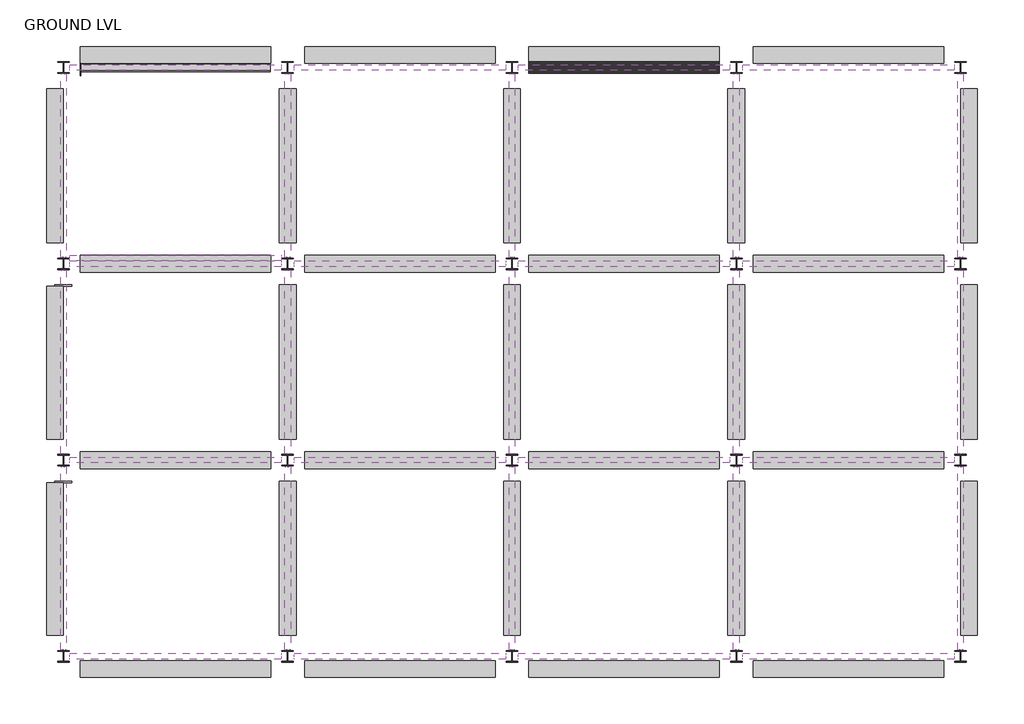
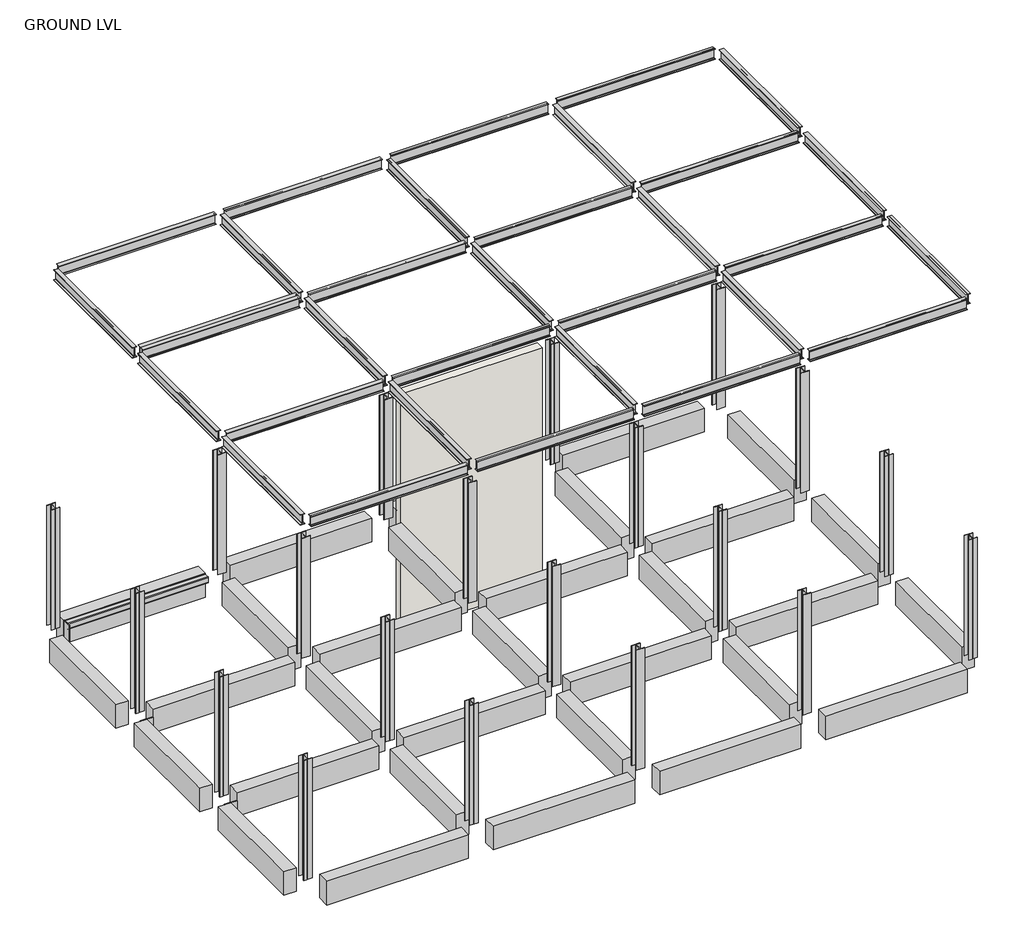
# One storey: 67 beams, 20 columns, 1 wall.
"""IFC4 building model written with IfcOpenShell, lengths in millimetres."""

from ifc_helpers import new_model, si_unit, frame, origin, place, context, project, spatial, polyline, outline, extrude, faceted_brep, transform, mapped, element, save
from components import m_hss_square_hss152_4x152_4x9_5_4d3a2309, ub_universal_beams_ub254x102x28_022e5764, ub_universal_beams_ub254x102x28_3359efaf, ub_universal_beams_ub254x102x28_3001bc84, uc_universal_columns_column_uc203x203x52_f24fe326

model = new_model("IFC4")

# Units and contexts
model_context = context("Model", 3, world=origin())
ifc_project = project(units=[si_unit("LENGTHUNIT", "METRE", prefix="MILLI")], contexts=[model_context])

# Site, building, storey
site = spatial("IfcSite", under=ifc_project)
building = spatial("IfcBuilding", under=site)
storey = spatial("IfcBuildingStorey", under=building, Name="GROUND LVL", Elevation=0.0)

# Beams
placement = place(None, origin())
element("IfcBeam", 1, ObjectType="M_Concrete-Rectangular Beam : 300 x 600mm", at=placement, inside=storey, context=model_context, shape_type="Brep", body=[
    faceted_brep([(-5230.6620752, 9930.8028699, 0.0), (-5230.6620752, 10230.8028699, 0.0), (-8630.6620752, 10230.8028699, 0.0), (-8630.6620752, 9930.8028699, 0.0), (-8617.9620752, 9930.8028699, 0.0), (-5230.6620752, 9930.8028699, -600.0), (-8630.6620752, 9930.8028699, -600.0), (-8617.9620752, 9930.8028699, -600.0), (-5230.6620752, 10230.8028699, -600.0), (-8630.6620752, 10230.8028699, -600.0)], [[[0, 1, 2, 3, 4]], [[5, 0, 4, 3, 6, 7]], [[8, 5, 7, 6, 9]], [[1, 8, 9, 2]], [[2, 9, 6, 3]], [[1, 0, 5, 8]]]),
])
element("IfcBeam", 2, ObjectType="M_Concrete-Rectangular Beam : 300 x 600mm", at=placement, inside=storey, context=model_context, shape_type="SweptSolid", body=[
    extrude(outline(polyline([(-1230.6620752, 10230.8028699), (-1230.6620752, 9930.8028699), (-4630.6620752, 9930.8028699), (-4630.6620752, 10230.8028699), (-1230.6620752, 10230.8028699)])), frame((0.0, 0.0, -600.0), z_axis=(0.0, 0.0, 1.0), x_axis=(1.0, 0.0, 0.0)), (0.0, 0.0, 1.0), 600.0),
])
element("IfcBeam", 3, ObjectType="M_Concrete-Rectangular Beam : 300 x 600mm", at=placement, inside=storey, context=model_context, shape_type="SweptSolid", body=[
    extrude(outline(polyline([(-8930.6620752, 6730.8028699), (-9230.6620752, 6730.8028699), (-9230.6620752, 9480.8028699), (-8930.6620752, 9480.8028699), (-8930.6620752, 6730.8028699)])), frame((0.0, 0.0, -600.0), z_axis=(0.0, 0.0, 1.0), x_axis=(1.0, 0.0, 0.0)), (0.0, 0.0, 1.0), 600.0),
])
element("IfcBeam", 4, ObjectType="M_Concrete-Rectangular Beam : 300 x 600mm", at=placement, inside=storey, context=model_context, shape_type="Brep", body=[
    faceted_brep([(-9230.6620752, 3230.8028699, 0.0), (-8930.6620752, 3230.8028699, 0.0), (-8930.6620752, 5955.8028699, 0.0), (-9080.6620752, 5955.8028699, 0.0), (-9230.6620752, 5955.8028699, 0.0), (-9230.6620752, 3230.8028699, -600.0), (-9230.6620752, 5955.8028699, -600.0), (-8930.6620752, 3230.8028699, -600.0), (-9080.6620752, 5955.8028699, -600.0), (-8930.6620752, 5955.8028699, -600.0)], [[[0, 1, 2, 3, 4]], [[5, 0, 4, 6]], [[7, 5, 6, 8, 9]], [[1, 7, 9, 2]], [[2, 9, 8, 6, 4, 3]], [[1, 0, 5, 7]]]),
])
element("IfcBeam", 5, ObjectType="M_Concrete-Rectangular Beam : 300 x 600mm", at=placement, inside=storey, context=model_context, shape_type="Brep", body=[
    faceted_brep([(-9230.6620752, -269.1971301, 0.0), (-8930.6620752, -269.1971301, 0.0), (-8930.6620752, 2455.8028699, 0.0), (-9080.6620752, 2455.8028699, 0.0), (-9230.6620752, 2455.8028699, 0.0), (-9230.6620752, -269.1971301, -600.0), (-9230.6620752, 2455.8028699, -600.0), (-8930.6620752, -269.1971301, -600.0), (-9080.6620752, 2455.8028699, -600.0), (-8930.6620752, 2455.8028699, -600.0)], [[[0, 1, 2, 3, 4]], [[5, 0, 4, 6]], [[7, 5, 6, 8, 9]], [[1, 7, 9, 2]], [[2, 9, 8, 6, 4, 3]], [[1, 0, 5, 7]]]),
])
element("IfcBeam", 6, ObjectType="M_Concrete-Rectangular Beam : 300 x 600mm", at=placement, inside=storey, context=model_context, shape_type="Brep", body=[
    faceted_brep([(-9080.6620752, 2455.8028699, 0.0), (-8930.6620752, 2455.8028699, 0.0), (-8780.6620752, 2455.8028699, 0.0), (-8780.6620752, 2480.8028699, 0.0), (-9080.6620752, 2480.8028699, 0.0), (-8780.6620752, 2455.8028699, -600.0), (-8780.6620752, 2480.8028699, -600.0), (-8930.6620752, 2455.8028699, -600.0), (-9080.6620752, 2455.8028699, -600.0), (-9080.6620752, 2480.8028699, -600.0)], [[[0, 1, 2, 3, 4]], [[2, 5, 6, 3]], [[5, 7, 8, 9, 6]], [[8, 0, 4, 9]], [[0, 8, 7, 5, 2, 1]], [[4, 3, 6, 9]]]),
])
element("IfcBeam", 7, ObjectType="M_Concrete-Rectangular Beam : 300 x 600mm", at=placement, inside=storey, context=model_context, shape_type="Brep", body=[
    faceted_brep([(-9080.6620752, 5955.8028699, 0.0), (-8930.6620752, 5955.8028699, 0.0), (-8780.6620752, 5955.8028699, 0.0), (-8780.6620752, 5980.8028699, 0.0), (-9080.6620752, 5980.8028699, 0.0), (-8780.6620752, 5955.8028699, -600.0), (-8780.6620752, 5980.8028699, -600.0), (-8930.6620752, 5955.8028699, -600.0), (-9080.6620752, 5955.8028699, -600.0), (-9080.6620752, 5980.8028699, -600.0)], [[[0, 1, 2, 3, 4]], [[2, 5, 6, 3]], [[5, 7, 8, 9, 6]], [[8, 0, 4, 9]], [[0, 8, 7, 5, 2, 1]], [[4, 3, 6, 9]]]),
])
element("IfcBeam", 8, ObjectType="M_Concrete-Rectangular Beam : 300 x 600mm", at=placement, inside=storey, context=model_context, shape_type="SweptSolid", body=[
    extrude(outline(polyline([(-5080.6620752, 2480.8028699), (-4780.6620752, 2480.8028699), (-4780.6620752, -269.1971301), (-5080.6620752, -269.1971301), (-5080.6620752, 2480.8028699)])), frame((0.0, 0.0, -600.0), z_axis=(0.0, 0.0, 1.0), x_axis=(1.0, 0.0, 0.0)), (0.0, 0.0, 1.0), 600.0),
])
element("IfcBeam", 9, ObjectType="M_Concrete-Rectangular Beam : 300 x 600mm", at=placement, inside=storey, context=model_context, shape_type="SweptSolid", body=[
    extrude(outline(polyline([(-5080.6620752, 5980.8028699), (-4780.6620752, 5980.8028699), (-4780.6620752, 3230.8028699), (-5080.6620752, 3230.8028699), (-5080.6620752, 5980.8028699)])), frame((0.0, 0.0, -600.0), z_axis=(0.0, 0.0, 1.0), x_axis=(1.0, 0.0, 0.0)), (0.0, 0.0, 1.0), 600.0),
])
element("IfcBeam", 10, ObjectType="M_Concrete-Rectangular Beam : 300 x 600mm", at=placement, inside=storey, context=model_context, shape_type="SweptSolid", body=[
    extrude(outline(polyline([(-5080.6620752, 9480.8028699), (-4780.6620752, 9480.8028699), (-4780.6620752, 6730.8028699), (-5080.6620752, 6730.8028699), (-5080.6620752, 9480.8028699)])), frame((0.0, 0.0, -600.0), z_axis=(0.0, 0.0, 1.0), x_axis=(1.0, 0.0, 0.0)), (0.0, 0.0, 1.0), 600.0),
])
element("IfcBeam", 11, ObjectType="M_Concrete-Rectangular Beam : 300 x 600mm", at=placement, inside=storey, context=model_context, shape_type="SweptSolid", body=[
    extrude(outline(polyline([(-1080.6620752, 2480.8028699), (-780.6620752, 2480.8028699), (-780.6620752, -269.1971301), (-1080.6620752, -269.1971301), (-1080.6620752, 2480.8028699)])), frame((0.0, 0.0, -600.0), z_axis=(0.0, 0.0, 1.0), x_axis=(1.0, 0.0, 0.0)), (0.0, 0.0, 1.0), 600.0),
])
element("IfcBeam", 12, ObjectType="M_Concrete-Rectangular Beam : 300 x 600mm", at=placement, inside=storey, context=model_context, shape_type="SweptSolid", body=[
    extrude(outline(polyline([(-1080.6620752, 5980.8028699), (-780.6620752, 5980.8028699), (-780.6620752, 3230.8028699), (-1080.6620752, 3230.8028699), (-1080.6620752, 5980.8028699)])), frame((0.0, 0.0, -600.0), z_axis=(0.0, 0.0, 1.0), x_axis=(1.0, 0.0, 0.0)), (0.0, 0.0, 1.0), 600.0),
])
element("IfcBeam", 13, ObjectType="M_Concrete-Rectangular Beam : 300 x 600mm", at=placement, inside=storey, context=model_context, shape_type="SweptSolid", body=[
    extrude(outline(polyline([(-1080.6620752, 9480.8028699), (-780.6620752, 9480.8028699), (-780.6620752, 6730.8028699), (-1080.6620752, 6730.8028699), (-1080.6620752, 9480.8028699)])), frame((0.0, 0.0, -600.0), z_axis=(0.0, 0.0, 1.0), x_axis=(1.0, 0.0, 0.0)), (0.0, 0.0, 1.0), 600.0),
])
element("IfcBeam", 14, ObjectType="M_Concrete-Rectangular Beam : 300 x 600mm", at=placement, inside=storey, context=model_context, shape_type="SweptSolid", body=[
    extrude(outline(polyline([(2919.3379248, 2480.8028699), (3219.3379248, 2480.8028699), (3219.3379248, -269.1971301), (2919.3379248, -269.1971301), (2919.3379248, 2480.8028699)])), frame((0.0, 0.0, -600.0), z_axis=(0.0, 0.0, 1.0), x_axis=(1.0, 0.0, 0.0)), (0.0, 0.0, 1.0), 600.0),
])
element("IfcBeam", 15, ObjectType="M_Concrete-Rectangular Beam : 300 x 600mm", at=placement, inside=storey, context=model_context, shape_type="SweptSolid", body=[
    extrude(outline(polyline([(2919.3379248, 5980.8028699), (3219.3379248, 5980.8028699), (3219.3379248, 3230.8028699), (2919.3379248, 3230.8028699), (2919.3379248, 5980.8028699)])), frame((0.0, 0.0, -600.0), z_axis=(0.0, 0.0, 1.0), x_axis=(1.0, 0.0, 0.0)), (0.0, 0.0, 1.0), 600.0),
])
element("IfcBeam", 16, ObjectType="M_Concrete-Rectangular Beam : 300 x 600mm", at=placement, inside=storey, context=model_context, shape_type="SweptSolid", body=[
    extrude(outline(polyline([(2919.3379248, 9480.8028699), (3219.3379248, 9480.8028699), (3219.3379248, 6730.8028699), (2919.3379248, 6730.8028699), (2919.3379248, 9480.8028699)])), frame((0.0, 0.0, -600.0), z_axis=(0.0, 0.0, 1.0), x_axis=(1.0, 0.0, 0.0)), (0.0, 0.0, 1.0), 600.0),
])
element("IfcBeam", 17, ObjectType="M_Concrete-Rectangular Beam : 300 x 600mm", at=placement, inside=storey, context=model_context, shape_type="SweptSolid", body=[
    extrude(outline(polyline([(7069.3379248, 2480.8028699), (7369.3379248, 2480.8028699), (7369.3379248, -269.1971301), (7069.3379248, -269.1971301), (7069.3379248, 2480.8028699)])), frame((0.0, 0.0, -600.0), z_axis=(0.0, 0.0, 1.0), x_axis=(1.0, 0.0, 0.0)), (0.0, 0.0, 1.0), 600.0),
])
element("IfcBeam", 18, ObjectType="M_Concrete-Rectangular Beam : 300 x 600mm", at=placement, inside=storey, context=model_context, shape_type="SweptSolid", body=[
    extrude(outline(polyline([(7069.3379248, 5980.8028699), (7369.3379248, 5980.8028699), (7369.3379248, 3230.8028699), (7069.3379248, 3230.8028699), (7069.3379248, 5980.8028699)])), frame((0.0, 0.0, -600.0), z_axis=(0.0, 0.0, 1.0), x_axis=(1.0, 0.0, 0.0)), (0.0, 0.0, 1.0), 600.0),
])
element("IfcBeam", 19, ObjectType="M_Concrete-Rectangular Beam : 300 x 600mm", at=placement, inside=storey, context=model_context, shape_type="SweptSolid", body=[
    extrude(outline(polyline([(7069.3379248, 9480.8028699), (7369.3379248, 9480.8028699), (7369.3379248, 6730.8028699), (7069.3379248, 6730.8028699), (7069.3379248, 9480.8028699)])), frame((0.0, 0.0, -600.0), z_axis=(0.0, 0.0, 1.0), x_axis=(1.0, 0.0, 0.0)), (0.0, 0.0, 1.0), 600.0),
])
element("IfcBeam", 20, ObjectType="M_Concrete-Rectangular Beam : 300 x 600mm", at=placement, inside=storey, context=model_context, shape_type="SweptSolid", body=[
    extrude(outline(polyline([(-8630.6620752, 9930.8028699), (-8617.9620752, 9930.8028699), (-8617.9620752, 9705.8028699), (-8630.6620752, 9705.8028699), (-8630.6620752, 9930.8028699)])), frame((0.0, 0.0, -600.0), z_axis=(0.0, 0.0, 1.0), x_axis=(1.0, 0.0, 0.0)), (0.0, 0.0, 1.0), 600.0),
])
element("IfcBeam", 21, ObjectType="M_Concrete-Rectangular Beam : 300 x 600mm", at=placement, inside=storey, context=model_context, shape_type="SweptSolid", body=[
    extrude(outline(polyline([(-630.6620752, 9930.8028699), (-630.6620752, 10230.8028699), (2769.3379248, 10230.8028699), (2769.3379248, 9930.8028699), (-630.6620752, 9930.8028699)])), frame((0.0, 0.0, -600.0), z_axis=(0.0, 0.0, 1.0), x_axis=(1.0, 0.0, 0.0)), (0.0, 0.0, 1.0), 600.0),
])
element("IfcBeam", 22, ObjectType="M_Concrete-Rectangular Beam : 300 x 600mm", at=placement, inside=storey, context=model_context, shape_type="SweptSolid", body=[
    extrude(outline(polyline([(3369.3379248, 9930.8028699), (3369.3379248, 10230.8028699), (6769.3379248, 10230.8028699), (6769.3379248, 9930.8028699), (3369.3379248, 9930.8028699)])), frame((0.0, 0.0, -600.0), z_axis=(0.0, 0.0, 1.0), x_axis=(1.0, 0.0, 0.0)), (0.0, 0.0, 1.0), 600.0),
])
element("IfcBeam", 23, ObjectType="M_Concrete-Rectangular Beam : 300 x 600mm", at=placement, inside=storey, context=model_context, shape_type="SweptSolid", body=[
    extrude(outline(polyline([(-8630.6620752, 6205.8028699), (-8630.6620752, 6505.8028699), (-5230.6620752, 6505.8028699), (-5230.6620752, 6205.8028699), (-8630.6620752, 6205.8028699)])), frame((0.0, 0.0, -600.0), z_axis=(0.0, 0.0, 1.0), x_axis=(1.0, 0.0, 0.0)), (0.0, 0.0, 1.0), 600.0),
])
element("IfcBeam", 24, ObjectType="M_Concrete-Rectangular Beam : 300 x 600mm", at=placement, inside=storey, context=model_context, shape_type="SweptSolid", body=[
    extrude(outline(polyline([(-4630.6620752, 6205.8028699), (-4630.6620752, 6505.8028699), (-1230.6620752, 6505.8028699), (-1230.6620752, 6205.8028699), (-4630.6620752, 6205.8028699)])), frame((0.0, 0.0, -600.0), z_axis=(0.0, 0.0, 1.0), x_axis=(1.0, 0.0, 0.0)), (0.0, 0.0, 1.0), 600.0),
])
element("IfcBeam", 25, ObjectType="M_Concrete-Rectangular Beam : 300 x 600mm", at=placement, inside=storey, context=model_context, shape_type="SweptSolid", body=[
    extrude(outline(polyline([(-630.6620752, 6205.8028699), (-630.6620752, 6505.8028699), (2769.3379248, 6505.8028699), (2769.3379248, 6205.8028699), (-630.6620752, 6205.8028699)])), frame((0.0, 0.0, -600.0), z_axis=(0.0, 0.0, 1.0), x_axis=(1.0, 0.0, 0.0)), (0.0, 0.0, 1.0), 600.0),
])
element("IfcBeam", 26, ObjectType="M_Concrete-Rectangular Beam : 300 x 600mm", at=placement, inside=storey, context=model_context, shape_type="SweptSolid", body=[
    extrude(outline(polyline([(3369.3379248, 6205.8028699), (3369.3379248, 6505.8028699), (6769.3379248, 6505.8028699), (6769.3379248, 6205.8028699), (3369.3379248, 6205.8028699)])), frame((0.0, 0.0, -600.0), z_axis=(0.0, 0.0, 1.0), x_axis=(1.0, 0.0, 0.0)), (0.0, 0.0, 1.0), 600.0),
])
element("IfcBeam", 27, ObjectType="M_Concrete-Rectangular Beam : 300 x 600mm", at=placement, inside=storey, context=model_context, shape_type="SweptSolid", body=[
    extrude(outline(polyline([(-8630.6620752, 2705.8028699), (-8630.6620752, 3005.8028699), (-5230.6620752, 3005.8028699), (-5230.6620752, 2705.8028699), (-8630.6620752, 2705.8028699)])), frame((0.0, 0.0, -600.0), z_axis=(0.0, 0.0, 1.0), x_axis=(1.0, 0.0, 0.0)), (0.0, 0.0, 1.0), 600.0),
])
element("IfcBeam", 28, ObjectType="M_Concrete-Rectangular Beam : 300 x 600mm", at=placement, inside=storey, context=model_context, shape_type="SweptSolid", body=[
    extrude(outline(polyline([(-4630.6620752, 2705.8028699), (-4630.6620752, 3005.8028699), (-1230.6620752, 3005.8028699), (-1230.6620752, 2705.8028699), (-4630.6620752, 2705.8028699)])), frame((0.0, 0.0, -600.0), z_axis=(0.0, 0.0, 1.0), x_axis=(1.0, 0.0, 0.0)), (0.0, 0.0, 1.0), 600.0),
])
element("IfcBeam", 29, ObjectType="M_Concrete-Rectangular Beam : 300 x 600mm", at=placement, inside=storey, context=model_context, shape_type="SweptSolid", body=[
    extrude(outline(polyline([(-630.6620752, 2705.8028699), (-630.6620752, 3005.8028699), (2769.3379248, 3005.8028699), (2769.3379248, 2705.8028699), (-630.6620752, 2705.8028699)])), frame((0.0, 0.0, -600.0), z_axis=(0.0, 0.0, 1.0), x_axis=(1.0, 0.0, 0.0)), (0.0, 0.0, 1.0), 600.0),
])
element("IfcBeam", 30, ObjectType="M_Concrete-Rectangular Beam : 300 x 600mm", at=placement, inside=storey, context=model_context, shape_type="SweptSolid", body=[
    extrude(outline(polyline([(3369.3379248, 2705.8028699), (3369.3379248, 3005.8028699), (6769.3379248, 3005.8028699), (6769.3379248, 2705.8028699), (3369.3379248, 2705.8028699)])), frame((0.0, 0.0, -600.0), z_axis=(0.0, 0.0, 1.0), x_axis=(1.0, 0.0, 0.0)), (0.0, 0.0, 1.0), 600.0),
])
element("IfcBeam", 31, ObjectType="M_Concrete-Rectangular Beam : 300 x 600mm", at=placement, inside=storey, context=model_context, shape_type="SweptSolid", body=[
    extrude(outline(polyline([(-8630.6620752, -1019.1971301), (-8630.6620752, -719.1971301), (-5230.6620752, -719.1971301), (-5230.6620752, -1019.1971301), (-8630.6620752, -1019.1971301)])), frame((0.0, 0.0, -600.0), z_axis=(0.0, 0.0, 1.0), x_axis=(1.0, 0.0, 0.0)), (0.0, 0.0, 1.0), 600.0),
])
element("IfcBeam", 32, ObjectType="M_Concrete-Rectangular Beam : 300 x 600mm", at=placement, inside=storey, context=model_context, shape_type="SweptSolid", body=[
    extrude(outline(polyline([(-4630.6620752, -1019.1971301), (-4630.6620752, -719.1971301), (-1230.6620752, -719.1971301), (-1230.6620752, -1019.1971301), (-4630.6620752, -1019.1971301)])), frame((0.0, 0.0, -600.0), z_axis=(0.0, 0.0, 1.0), x_axis=(1.0, 0.0, 0.0)), (0.0, 0.0, 1.0), 600.0),
])
element("IfcBeam", 33, ObjectType="M_Concrete-Rectangular Beam : 300 x 600mm", at=placement, inside=storey, context=model_context, shape_type="SweptSolid", body=[
    extrude(outline(polyline([(-630.6620752, -1019.1971301), (-630.6620752, -719.1971301), (2769.3379248, -719.1971301), (2769.3379248, -1019.1971301), (-630.6620752, -1019.1971301)])), frame((0.0, 0.0, -600.0), z_axis=(0.0, 0.0, 1.0), x_axis=(1.0, 0.0, 0.0)), (0.0, 0.0, 1.0), 600.0),
])
element("IfcBeam", 34, ObjectType="M_Concrete-Rectangular Beam : 300 x 600mm", at=placement, inside=storey, context=model_context, shape_type="SweptSolid", body=[
    extrude(outline(polyline([(3369.3379248, -1019.1971301), (3369.3379248, -719.1971301), (6769.3379248, -719.1971301), (6769.3379248, -1019.1971301), (3369.3379248, -1019.1971301)])), frame((0.0, 0.0, -600.0), z_axis=(0.0, 0.0, 1.0), x_axis=(1.0, 0.0, 0.0)), (0.0, 0.0, 1.0), 600.0),
])
m_hss_square_hss152_4x152_4x9_5_shape = m_hss_square_hss152_4x152_4x9_5_4d3a2309(model_context)
element("IfcBeam", 35, ObjectType="M_HSS Square : HSS152.4X152.4X9.5", at=placement, inside=storey, context=model_context, shape_type="MappedRepresentation", body=[
    mapped(m_hss_square_hss152_4x152_4x9_5_shape, transform((-6880.6620752, 9855.8028699, -76.0), x_axis=(1.0, 0.0, 0.0), y_axis=(0.0, 1.0, 0.0), z_axis=(0.0, 0.0, 1.0))),
])
ub_universal_beams_ub254x102x28_shape = ub_universal_beams_ub254x102x28_022e5764(model_context)
element("IfcBeam", 36, ObjectType="UB-Universal Beams : UB254x102x28", at=placement, inside=storey, context=model_context, shape_type="MappedRepresentation", body=[
    mapped(ub_universal_beams_ub254x102x28_shape, transform((-6871.2144105, 6458.2567898, 9013.8), x_axis=(1.0, 0.0, 0.0), y_axis=(0.0, 1.0, 0.0), z_axis=(0.0, 0.0, 1.0))),
])
ub_universal_beams_ub254x102x28_2_shape = ub_universal_beams_ub254x102x28_3359efaf(model_context)
element("IfcBeam", 37, ObjectType="UB-Universal Beams : UB254x102x28", at=placement, inside=storey, context=model_context, shape_type="MappedRepresentation", body=[
    mapped(ub_universal_beams_ub254x102x28_2_shape, transform((-8930.6620752, 1105.8028699, 9013.8), x_axis=(0.0, 1.0, 0.0), y_axis=(-1.0, 0.0, 0.0), z_axis=(0.0, 0.0, 1.0))),
])
element("IfcBeam", 38, ObjectType="UB-Universal Beams : UB254x102x28", at=placement, inside=storey, context=model_context, shape_type="MappedRepresentation", body=[
    mapped(ub_universal_beams_ub254x102x28_2_shape, transform((-8930.6620752, 4605.8028699, 9013.8), x_axis=(0.0, 1.0, 0.0), y_axis=(-1.0, 0.0, 0.0), z_axis=(0.0, 0.0, 1.0))),
])
element("IfcBeam", 39, ObjectType="UB-Universal Beams : UB254x102x28", at=placement, inside=storey, context=model_context, shape_type="MappedRepresentation", body=[
    mapped(ub_universal_beams_ub254x102x28_2_shape, transform((-8930.6620752, 8105.8028699, 9013.8), x_axis=(0.0, 1.0, 0.0), y_axis=(-1.0, 0.0, 0.0), z_axis=(0.0, 0.0, 1.0))),
])
element("IfcBeam", 40, ObjectType="UB-Universal Beams : UB254x102x28", at=placement, inside=storey, context=model_context, shape_type="MappedRepresentation", body=[
    mapped(ub_universal_beams_ub254x102x28_2_shape, transform((-4930.6620752, 1105.8028699, 9013.8), x_axis=(0.0, 1.0, 0.0), y_axis=(-1.0, 0.0, 0.0), z_axis=(0.0, 0.0, 1.0))),
])
element("IfcBeam", 41, ObjectType="UB-Universal Beams : UB254x102x28", at=placement, inside=storey, context=model_context, shape_type="MappedRepresentation", body=[
    mapped(ub_universal_beams_ub254x102x28_2_shape, transform((-4930.6620752, 4605.8028699, 9013.8), x_axis=(0.0, 1.0, 0.0), y_axis=(-1.0, 0.0, 0.0), z_axis=(0.0, 0.0, 1.0))),
])
element("IfcBeam", 42, ObjectType="UB-Universal Beams : UB254x102x28", at=placement, inside=storey, context=model_context, shape_type="MappedRepresentation", body=[
    mapped(ub_universal_beams_ub254x102x28_2_shape, transform((-4930.6620752, 8105.8028699, 9013.8), x_axis=(0.0, 1.0, 0.0), y_axis=(-1.0, 0.0, 0.0), z_axis=(0.0, 0.0, 1.0))),
])
element("IfcBeam", 43, ObjectType="UB-Universal Beams : UB254x102x28", at=placement, inside=storey, context=model_context, shape_type="MappedRepresentation", body=[
    mapped(ub_universal_beams_ub254x102x28_2_shape, transform((-930.6620752, 1105.8028699, 9013.8), x_axis=(0.0, 1.0, 0.0), y_axis=(-1.0, 0.0, 0.0), z_axis=(0.0, 0.0, 1.0))),
])
element("IfcBeam", 44, ObjectType="UB-Universal Beams : UB254x102x28", at=placement, inside=storey, context=model_context, shape_type="MappedRepresentation", body=[
    mapped(ub_universal_beams_ub254x102x28_2_shape, transform((-930.6620752, 4605.8028699, 9013.8), x_axis=(0.0, 1.0, 0.0), y_axis=(-1.0, 0.0, 0.0), z_axis=(0.0, 0.0, 1.0))),
])
element("IfcBeam", 45, ObjectType="UB-Universal Beams : UB254x102x28", at=placement, inside=storey, context=model_context, shape_type="MappedRepresentation", body=[
    mapped(ub_universal_beams_ub254x102x28_2_shape, transform((-930.6620752, 8105.8028699, 9013.8), x_axis=(0.0, 1.0, 0.0), y_axis=(-1.0, 0.0, 0.0), z_axis=(0.0, 0.0, 1.0))),
])
element("IfcBeam", 46, ObjectType="UB-Universal Beams : UB254x102x28", at=placement, inside=storey, context=model_context, shape_type="MappedRepresentation", body=[
    mapped(ub_universal_beams_ub254x102x28_2_shape, transform((3069.3379248, 1105.8028699, 9013.8), x_axis=(0.0, 1.0, 0.0), y_axis=(-1.0, 0.0, 0.0), z_axis=(0.0, 0.0, 1.0))),
])
element("IfcBeam", 47, ObjectType="UB-Universal Beams : UB254x102x28", at=placement, inside=storey, context=model_context, shape_type="MappedRepresentation", body=[
    mapped(ub_universal_beams_ub254x102x28_2_shape, transform((3069.3379248, 4605.8028699, 9013.8), x_axis=(0.0, 1.0, 0.0), y_axis=(-1.0, 0.0, 0.0), z_axis=(0.0, 0.0, 1.0))),
])
element("IfcBeam", 48, ObjectType="UB-Universal Beams : UB254x102x28", at=placement, inside=storey, context=model_context, shape_type="MappedRepresentation", body=[
    mapped(ub_universal_beams_ub254x102x28_2_shape, transform((3069.3379248, 8105.8028699, 9013.8), x_axis=(0.0, 1.0, 0.0), y_axis=(-1.0, 0.0, 0.0), z_axis=(0.0, 0.0, 1.0))),
])
element("IfcBeam", 49, ObjectType="UB-Universal Beams : UB254x102x28", at=placement, inside=storey, context=model_context, shape_type="MappedRepresentation", body=[
    mapped(ub_universal_beams_ub254x102x28_2_shape, transform((7069.3379248, 1105.8028699, 9013.8), x_axis=(0.0, 1.0, 0.0), y_axis=(-1.0, 0.0, 0.0), z_axis=(0.0, 0.0, 1.0))),
])
element("IfcBeam", 50, ObjectType="UB-Universal Beams : UB254x102x28", at=placement, inside=storey, context=model_context, shape_type="MappedRepresentation", body=[
    mapped(ub_universal_beams_ub254x102x28_2_shape, transform((7069.3379248, 4605.8028699, 9013.8), x_axis=(0.0, 1.0, 0.0), y_axis=(-1.0, 0.0, 0.0), z_axis=(0.0, 0.0, 1.0))),
])
element("IfcBeam", 51, ObjectType="UB-Universal Beams : UB254x102x28", at=placement, inside=storey, context=model_context, shape_type="MappedRepresentation", body=[
    mapped(ub_universal_beams_ub254x102x28_2_shape, transform((7069.3379248, 8105.8028699, 9013.8), x_axis=(0.0, 1.0, 0.0), y_axis=(-1.0, 0.0, 0.0), z_axis=(0.0, 0.0, 1.0))),
])
ub_universal_beams_ub254x102x28_3_shape = ub_universal_beams_ub254x102x28_3001bc84(model_context)
element("IfcBeam", 52, ObjectType="UB-Universal Beams : UB254x102x28", at=placement, inside=storey, context=model_context, shape_type="MappedRepresentation", body=[
    mapped(ub_universal_beams_ub254x102x28_3_shape, transform((-6930.6620752, 9855.8028699, 9013.8), x_axis=(1.0, 0.0, 0.0), y_axis=(0.0, 1.0, 0.0), z_axis=(0.0, 0.0, 1.0))),
])
element("IfcBeam", 53, ObjectType="UB-Universal Beams : UB254x102x28", at=placement, inside=storey, context=model_context, shape_type="MappedRepresentation", body=[
    mapped(ub_universal_beams_ub254x102x28_3_shape, transform((-2930.6620752, 9855.8028699, 9013.8), x_axis=(1.0, 0.0, 0.0), y_axis=(0.0, 1.0, 0.0), z_axis=(0.0, 0.0, 1.0))),
])
element("IfcBeam", 54, ObjectType="UB-Universal Beams : UB254x102x28", at=placement, inside=storey, context=model_context, shape_type="MappedRepresentation", body=[
    mapped(ub_universal_beams_ub254x102x28_3_shape, transform((1069.3379248, 9855.8028699, 9013.8), x_axis=(1.0, 0.0, 0.0), y_axis=(0.0, 1.0, 0.0), z_axis=(0.0, 0.0, 1.0))),
])
element("IfcBeam", 55, ObjectType="UB-Universal Beams : UB254x102x28", at=placement, inside=storey, context=model_context, shape_type="MappedRepresentation", body=[
    mapped(ub_universal_beams_ub254x102x28_3_shape, transform((5069.3379248, 9855.8028699, 9013.8), x_axis=(1.0, 0.0, 0.0), y_axis=(0.0, 1.0, 0.0), z_axis=(0.0, 0.0, 1.0))),
])
element("IfcBeam", 56, ObjectType="UB-Universal Beams : UB254x102x28", at=placement, inside=storey, context=model_context, shape_type="MappedRepresentation", body=[
    mapped(ub_universal_beams_ub254x102x28_3_shape, transform((-6930.6620752, 6355.8028699, 9013.8), x_axis=(1.0, 0.0, 0.0), y_axis=(0.0, 1.0, 0.0), z_axis=(0.0, 0.0, 1.0))),
])
element("IfcBeam", 57, ObjectType="UB-Universal Beams : UB254x102x28", at=placement, inside=storey, context=model_context, shape_type="MappedRepresentation", body=[
    mapped(ub_universal_beams_ub254x102x28_3_shape, transform((-2930.6620752, 6355.8028699, 9013.8), x_axis=(1.0, 0.0, 0.0), y_axis=(0.0, 1.0, 0.0), z_axis=(0.0, 0.0, 1.0))),
])
element("IfcBeam", 58, ObjectType="UB-Universal Beams : UB254x102x28", at=placement, inside=storey, context=model_context, shape_type="MappedRepresentation", body=[
    mapped(ub_universal_beams_ub254x102x28_3_shape, transform((1069.3379248, 6355.8028699, 9013.8), x_axis=(1.0, 0.0, 0.0), y_axis=(0.0, 1.0, 0.0), z_axis=(0.0, 0.0, 1.0))),
])
element("IfcBeam", 59, ObjectType="UB-Universal Beams : UB254x102x28", at=placement, inside=storey, context=model_context, shape_type="MappedRepresentation", body=[
    mapped(ub_universal_beams_ub254x102x28_3_shape, transform((5069.3379248, 6355.8028699, 9013.8), x_axis=(1.0, 0.0, 0.0), y_axis=(0.0, 1.0, 0.0), z_axis=(0.0, 0.0, 1.0))),
])
element("IfcBeam", 60, ObjectType="UB-Universal Beams : UB254x102x28", at=placement, inside=storey, context=model_context, shape_type="MappedRepresentation", body=[
    mapped(ub_universal_beams_ub254x102x28_3_shape, transform((-6930.6620752, 2855.8028699, 9013.8), x_axis=(1.0, 0.0, 0.0), y_axis=(0.0, 1.0, 0.0), z_axis=(0.0, 0.0, 1.0))),
])
element("IfcBeam", 61, ObjectType="UB-Universal Beams : UB254x102x28", at=placement, inside=storey, context=model_context, shape_type="MappedRepresentation", body=[
    mapped(ub_universal_beams_ub254x102x28_3_shape, transform((-2930.6620752, 2855.8028699, 9013.8), x_axis=(1.0, 0.0, 0.0), y_axis=(0.0, 1.0, 0.0), z_axis=(0.0, 0.0, 1.0))),
])
element("IfcBeam", 62, ObjectType="UB-Universal Beams : UB254x102x28", at=placement, inside=storey, context=model_context, shape_type="MappedRepresentation", body=[
    mapped(ub_universal_beams_ub254x102x28_3_shape, transform((1069.3379248, 2855.8028699, 9013.8), x_axis=(1.0, 0.0, 0.0), y_axis=(0.0, 1.0, 0.0), z_axis=(0.0, 0.0, 1.0))),
])
element("IfcBeam", 63, ObjectType="UB-Universal Beams : UB254x102x28", at=placement, inside=storey, context=model_context, shape_type="MappedRepresentation", body=[
    mapped(ub_universal_beams_ub254x102x28_3_shape, transform((5069.3379248, 2855.8028699, 9013.8), x_axis=(1.0, 0.0, 0.0), y_axis=(0.0, 1.0, 0.0), z_axis=(0.0, 0.0, 1.0))),
])
element("IfcBeam", 64, ObjectType="UB-Universal Beams : UB254x102x28", at=placement, inside=storey, context=model_context, shape_type="MappedRepresentation", body=[
    mapped(ub_universal_beams_ub254x102x28_3_shape, transform((-6930.6620752, -644.1971301, 9013.8), x_axis=(1.0, 0.0, 0.0), y_axis=(0.0, 1.0, 0.0), z_axis=(0.0, 0.0, 1.0))),
])
element("IfcBeam", 65, ObjectType="UB-Universal Beams : UB254x102x28", at=placement, inside=storey, context=model_context, shape_type="MappedRepresentation", body=[
    mapped(ub_universal_beams_ub254x102x28_3_shape, transform((-2930.6620752, -644.1971301, 9013.8), x_axis=(1.0, 0.0, 0.0), y_axis=(0.0, 1.0, 0.0), z_axis=(0.0, 0.0, 1.0))),
])
element("IfcBeam", 66, ObjectType="UB-Universal Beams : UB254x102x28", at=placement, inside=storey, context=model_context, shape_type="MappedRepresentation", body=[
    mapped(ub_universal_beams_ub254x102x28_3_shape, transform((1069.3379248, -644.1971301, 9013.8), x_axis=(1.0, 0.0, 0.0), y_axis=(0.0, 1.0, 0.0), z_axis=(0.0, 0.0, 1.0))),
])
element("IfcBeam", 67, ObjectType="UB-Universal Beams : UB254x102x28", at=placement, inside=storey, context=model_context, shape_type="MappedRepresentation", body=[
    mapped(ub_universal_beams_ub254x102x28_3_shape, transform((5069.3379248, -644.1971301, 9013.8), x_axis=(1.0, 0.0, 0.0), y_axis=(0.0, 1.0, 0.0), z_axis=(0.0, 0.0, 1.0))),
])

# Columns
uc_universal_columns_column_uc203x203x52_shape = uc_universal_columns_column_uc203x203x52_f24fe326(model_context)
element("IfcColumn", 68, ObjectType="UC-Universal Columns-Column : UC203x203x52", at=placement, inside=storey, context=model_context, shape_type="MappedRepresentation", body=[
    mapped(uc_universal_columns_column_uc203x203x52_shape, transform((-8930.6620752, 9855.8028699, 0.0), x_axis=(1.0, 0.0, 0.0), y_axis=(0.0, 1.0, 0.0), z_axis=(0.0, 0.0, 1.0))),
])
element("IfcColumn", 69, ObjectType="UC-Universal Columns-Column : UC203x203x52", at=placement, inside=storey, context=model_context, shape_type="MappedRepresentation", body=[
    mapped(uc_universal_columns_column_uc203x203x52_shape, transform((-8930.6620752, 6355.8028699, 0.0), x_axis=(1.0, 0.0, 0.0), y_axis=(0.0, 1.0, 0.0), z_axis=(0.0, 0.0, 1.0))),
])
element("IfcColumn", 70, ObjectType="UC-Universal Columns-Column : UC203x203x52", at=placement, inside=storey, context=model_context, shape_type="MappedRepresentation", body=[
    mapped(uc_universal_columns_column_uc203x203x52_shape, transform((-8930.6620752, 2855.8028699, 0.0), x_axis=(1.0, 0.0, 0.0), y_axis=(0.0, 1.0, 0.0), z_axis=(0.0, 0.0, 1.0))),
])
element("IfcColumn", 71, ObjectType="UC-Universal Columns-Column : UC203x203x52", at=placement, inside=storey, context=model_context, shape_type="MappedRepresentation", body=[
    mapped(uc_universal_columns_column_uc203x203x52_shape, transform((-8930.6620752, -644.1971301, 0.0), x_axis=(1.0, 0.0, 0.0), y_axis=(0.0, 1.0, 0.0), z_axis=(0.0, 0.0, 1.0))),
])
element("IfcColumn", 72, ObjectType="UC-Universal Columns-Column : UC203x203x52", at=placement, inside=storey, context=model_context, shape_type="MappedRepresentation", body=[
    mapped(uc_universal_columns_column_uc203x203x52_shape, transform((-4930.6620752, 9855.8028699, 0.0), x_axis=(1.0, 0.0, 0.0), y_axis=(0.0, 1.0, 0.0), z_axis=(0.0, 0.0, 1.0))),
])
element("IfcColumn", 73, ObjectType="UC-Universal Columns-Column : UC203x203x52", at=placement, inside=storey, context=model_context, shape_type="MappedRepresentation", body=[
    mapped(uc_universal_columns_column_uc203x203x52_shape, transform((-4930.6620752, 6355.8028699, 0.0), x_axis=(1.0, 0.0, 0.0), y_axis=(0.0, 1.0, 0.0), z_axis=(0.0, 0.0, 1.0))),
])
element("IfcColumn", 74, ObjectType="UC-Universal Columns-Column : UC203x203x52", at=placement, inside=storey, context=model_context, shape_type="MappedRepresentation", body=[
    mapped(uc_universal_columns_column_uc203x203x52_shape, transform((-4930.6620752, 2855.8028699, 0.0), x_axis=(1.0, 0.0, 0.0), y_axis=(0.0, 1.0, 0.0), z_axis=(0.0, 0.0, 1.0))),
])
element("IfcColumn", 75, ObjectType="UC-Universal Columns-Column : UC203x203x52", at=placement, inside=storey, context=model_context, shape_type="MappedRepresentation", body=[
    mapped(uc_universal_columns_column_uc203x203x52_shape, transform((-4930.6620752, -644.1971301, 0.0), x_axis=(1.0, 0.0, 0.0), y_axis=(0.0, 1.0, 0.0), z_axis=(0.0, 0.0, 1.0))),
])
element("IfcColumn", 76, ObjectType="UC-Universal Columns-Column : UC203x203x52", at=placement, inside=storey, context=model_context, shape_type="MappedRepresentation", body=[
    mapped(uc_universal_columns_column_uc203x203x52_shape, transform((-930.6620752, 9855.8028699, 0.0), x_axis=(1.0, 0.0, 0.0), y_axis=(0.0, 1.0, 0.0), z_axis=(0.0, 0.0, 1.0))),
])
element("IfcColumn", 77, ObjectType="UC-Universal Columns-Column : UC203x203x52", at=placement, inside=storey, context=model_context, shape_type="MappedRepresentation", body=[
    mapped(uc_universal_columns_column_uc203x203x52_shape, transform((-930.6620752, 6355.8028699, 0.0), x_axis=(1.0, 0.0, 0.0), y_axis=(0.0, 1.0, 0.0), z_axis=(0.0, 0.0, 1.0))),
])
element("IfcColumn", 78, ObjectType="UC-Universal Columns-Column : UC203x203x52", at=placement, inside=storey, context=model_context, shape_type="MappedRepresentation", body=[
    mapped(uc_universal_columns_column_uc203x203x52_shape, transform((-930.6620752, 2855.8028699, 0.0), x_axis=(1.0, 0.0, 0.0), y_axis=(0.0, 1.0, 0.0), z_axis=(0.0, 0.0, 1.0))),
])
element("IfcColumn", 79, ObjectType="UC-Universal Columns-Column : UC203x203x52", at=placement, inside=storey, context=model_context, shape_type="MappedRepresentation", body=[
    mapped(uc_universal_columns_column_uc203x203x52_shape, transform((-930.6620752, -644.1971301, 0.0), x_axis=(1.0, 0.0, 0.0), y_axis=(0.0, 1.0, 0.0), z_axis=(0.0, 0.0, 1.0))),
])
element("IfcColumn", 80, ObjectType="UC-Universal Columns-Column : UC203x203x52", at=placement, inside=storey, context=model_context, shape_type="MappedRepresentation", body=[
    mapped(uc_universal_columns_column_uc203x203x52_shape, transform((3069.3379248, 9855.8028699, 0.0), x_axis=(1.0, 0.0, 0.0), y_axis=(0.0, 1.0, 0.0), z_axis=(0.0, 0.0, 1.0))),
])
element("IfcColumn", 81, ObjectType="UC-Universal Columns-Column : UC203x203x52", at=placement, inside=storey, context=model_context, shape_type="MappedRepresentation", body=[
    mapped(uc_universal_columns_column_uc203x203x52_shape, transform((3069.3379248, 6355.8028699, 0.0), x_axis=(1.0, 0.0, 0.0), y_axis=(0.0, 1.0, 0.0), z_axis=(0.0, 0.0, 1.0))),
])
element("IfcColumn", 82, ObjectType="UC-Universal Columns-Column : UC203x203x52", at=placement, inside=storey, context=model_context, shape_type="MappedRepresentation", body=[
    mapped(uc_universal_columns_column_uc203x203x52_shape, transform((3069.3379248, 2855.8028699, 0.0), x_axis=(1.0, 0.0, 0.0), y_axis=(0.0, 1.0, 0.0), z_axis=(0.0, 0.0, 1.0))),
])
element("IfcColumn", 83, ObjectType="UC-Universal Columns-Column : UC203x203x52", at=placement, inside=storey, context=model_context, shape_type="MappedRepresentation", body=[
    mapped(uc_universal_columns_column_uc203x203x52_shape, transform((3069.3379248, -644.1971301, 0.0), x_axis=(1.0, 0.0, 0.0), y_axis=(0.0, 1.0, 0.0), z_axis=(0.0, 0.0, 1.0))),
])
element("IfcColumn", 84, ObjectType="UC-Universal Columns-Column : UC203x203x52", at=placement, inside=storey, context=model_context, shape_type="MappedRepresentation", body=[
    mapped(uc_universal_columns_column_uc203x203x52_shape, transform((7069.3379248, 9855.8028699, 0.0), x_axis=(1.0, 0.0, 0.0), y_axis=(0.0, 1.0, 0.0), z_axis=(0.0, 0.0, 1.0))),
])
element("IfcColumn", 85, ObjectType="UC-Universal Columns-Column : UC203x203x52", at=placement, inside=storey, context=model_context, shape_type="MappedRepresentation", body=[
    mapped(uc_universal_columns_column_uc203x203x52_shape, transform((7069.3379248, 6355.8028699, 0.0), x_axis=(1.0, 0.0, 0.0), y_axis=(0.0, 1.0, 0.0), z_axis=(0.0, 0.0, 1.0))),
])
element("IfcColumn", 86, ObjectType="UC-Universal Columns-Column : UC203x203x52", at=placement, inside=storey, context=model_context, shape_type="MappedRepresentation", body=[
    mapped(uc_universal_columns_column_uc203x203x52_shape, transform((7069.3379248, 2855.8028699, 0.0), x_axis=(1.0, 0.0, 0.0), y_axis=(0.0, 1.0, 0.0), z_axis=(0.0, 0.0, 1.0))),
])
element("IfcColumn", 87, ObjectType="UC-Universal Columns-Column : UC203x203x52", at=placement, inside=storey, context=model_context, shape_type="MappedRepresentation", body=[
    mapped(uc_universal_columns_column_uc203x203x52_shape, transform((7069.3379248, -644.1971301, 0.0), x_axis=(1.0, 0.0, 0.0), y_axis=(0.0, 1.0, 0.0), z_axis=(0.0, 0.0, 1.0))),
])

# Wall
element("IfcWall", 88, ObjectType="Generic - 200mm", at=placement, inside=storey, context=model_context, shape_type="SweptSolid", body=[
    extrude(outline(polyline([(2769.3379248, 9755.8028699), (-630.6620752, 9755.8028699), (-630.6620752, 9955.8028699), (2769.3379248, 9955.8028699), (2769.3379248, 9755.8028699)])), frame((0.0, 0.0, -3000.0), z_axis=(0.0, 0.0, 1.0), x_axis=(1.0, 0.0, 0.0)), (0.0, 0.0, 1.0), 6048.0),
])

save(model, "model.ifc")

# Revit data of these elements
# Type "M_Concrete-Rectangular Beam : 300 x 600mm"
#   Length [instance default] = 5' - 0"
#   b = 0' - 11.81102"
#   h = 1' - 11.62205"
#   Structural Material [instance default] = Concrete, Cast-in-Place gray
#   Assembly Code = ""
# Type "M_HSS Square : HSS152.4X152.4X9.5"
#   Section Name Key = "HSS152.4X152.4X9.5"
#   Width = 15.2 cm
#   Wall Nominal Thickness = 0.953 cm
#   Wall Design Thickness = 0.886 cm
#   Torsional Moment of Inertia = 2690.00 cm⁴
#   Torsional Modulus = 362.0 cm³
#   Section Area = 48.9 cm²
#   Plastic Modulus weak axis = 259.0 cm³
#   Plastic Modulus strong axis = 259.0 cm³
#   Perimeter = 0.575 m²/m
#   Outer Fillet = 1.906 cm
#   Nominal Weight = 40.80 kgf/m
#   Moment of Inertia weak axis = 1640.00 cm⁴
#   Moment of Inertia strong axis = 1640.00 cm⁴
#   Length [instance default] = 5' - 0"
#   Inner Fillet = 0.953 cm
#   Height = 15.2 cm
#   Elastic Modulus weak axis = 216.0 cm³
#   Elastic Modulus strong axis = 216.0 cm³
#   Centroid Vertical = 7.6 cm
#   Centroid Horizontal = 7.6 cm
#   Structural Material [instance default] = Steel ASTM A500, Grade C, Rectangular and Square
# Type "UB-Universal Beams : UB254x102x28"
#   Section Name Key = "UB254X102X28"
#   Width = 10.22 cm
#   Web Thickness = 0.63 cm
#   Web Fillet = 0.76 cm
#   Warping Constant = 28000.0 cm⁶
#   Torsional Moment of Inertia = 9.57 cm⁴
#   Section Area = 36.1 cm²
#   Plastic Modulus weak axis = 54.8 cm³
#   Plastic Modulus strong axis = 353.0 cm³
#   Nominal Weight = 28.2999 kgf/m
#   Moment of Inertia weak axis = 179.00 cm⁴
#   Moment of Inertia strong axis = 4005.00 cm⁴
#   Height = 26.04 cm
#   Flange Thickness = 1.0 cm
#   Elastic Modulus weak axis = 34.9 cm³
#   Elastic Modulus strong axis = 308.0 cm³
#   Centroid Vertical = 13.02 cm
#   Centroid Horizontal = 5.11 cm
#   Bolt Spacing = 5.4 cm
#   Length [instance default] = 4' - 11.05512"
#   Structural Material [instance default] = Metal - Steel 43-275
#   Type Comments = ""
#   Assembly Code = ""
# Type "UC-Universal Columns-Column : UC203x203x52"
#   Section Name Key = "UC203x203x52"
#   Width = 20.43 cm
#   Web Thickness = 0.79 cm
#   Web Fillet = 1.02 cm
#   Warping Constant = 167000.0 cm⁶
#   Torsional Moment of Inertia = 31.80 cm⁴
#   Section Area = 66.0 cm²
#   Plastic Modulus weak axis = 264.0 cm³
#   Plastic Modulus strong axis = 567.0 cm³
#   Nominal Weight = 51.9998 kgf/m
#   Moment of Inertia weak axis = 1778.00 cm⁴
#   Moment of Inertia strong axis = 5259.00 cm⁴
#   Height = 20.62 cm
#   Flange Thickness = 1.25 cm
#   Elastic Modulus weak axis = 174.0 cm³
#   Elastic Modulus strong axis = 510.0 cm³
#   Centroid Vertical = 10.31 cm
#   Centroid Horizontal = 10.215 cm
#   Bolt Spacing = 14.0 cm
#   Structural Material [instance default] = Metal - Steel 43-275
#   Type Comments = ""
#   Assembly Code = ""
# Type "Generic - 200mm"
#   Layers, outside or top first: 0' - 7.87402" no material (function 1)
# Elements 1, 2, 3, 4, 5, 6, 7, 8, 9, 10, 11, 12, 13, 14, 15, 16, 17, 18, 19, 20, 21, 22, 23, 24, 25, 26, 27, 28, 29, 30, 31, 32, 33, 34 (IfcBeam, "M_Concrete-Rectangular Beam : 300 x 600mm")
#   Structural Material = Concrete, Cast-in-Place gray
#   Phase Created = New Construction
#   Materials on its faces: "Concrete, Cast-in-Place gray"
# Element 35 (IfcBeam, "M_HSS Square : HSS152.4X152.4X9.5")
#   Structural Material = Metal - Steel 43-275
#   Phase Created = New Construction
#   Materials on its faces: "Metal - Steel 43-275"
# Elements 36, 37, 38, 39, 40, 41, 42, 43, 44, 45, 46, 47, 48, 49, 50, 51, 52, 53, 54, 55, 56, 57, 58, 59, 60, 61, 62, 63, 64, 65, 66, 67 (IfcBeam, "UB-Universal Beams : UB254x102x28")
#   Structural Material = Metal - Steel 43-275
#   Phase Created = New Construction
#   Materials on its faces: "Metal - Steel 43-275"
# Elements 68, 69, 70, 71, 72, 73, 74, 75, 76, 77, 78, 79, 80, 81, 82, 83, 84, 85, 86, 87 (IfcColumn, "UC-Universal Columns-Column : UC203x203x52")
#   Structural Material = Metal - Steel 43-275
#   Phase Created = New Construction
#   Materials on its faces: "Metal - Steel 43-275"
# Element 88 (IfcWall, "Generic - 200mm")
#   built-in parameter 1001111 = -9' - 10.11024"
#   Top Offset = 0' - 0"
#   Base Offset = -9' - 10.11024"
#   wall height = 19' - 10.11024"
#   Phase Created = New Construction
#   Base Constraint = GROUND LVL
#   Top Constraint = FIRST FLOOR
#   Materials on its faces: "Default Wall"
# Materials
#   "Concrete, Cast-in-Place gray": class "Concrete", colour RGB 192 192 192, transparency 0, Description = "Cast-in-place concrete", Cost = 0
#   "Steel ASTM A500, Grade C, Rectangular and Square": class "Metal", colour RGB 120 120 120, transparency 0, Description = "Carbon steel", Cost = 0
#   "Metal - Steel 43-275": class "Metal", colour RGB 247 247 247, transparency 0, Cost = 0
#   "Default Wall": colour RGB 128 128 128, transparency 0, Cost = 0
